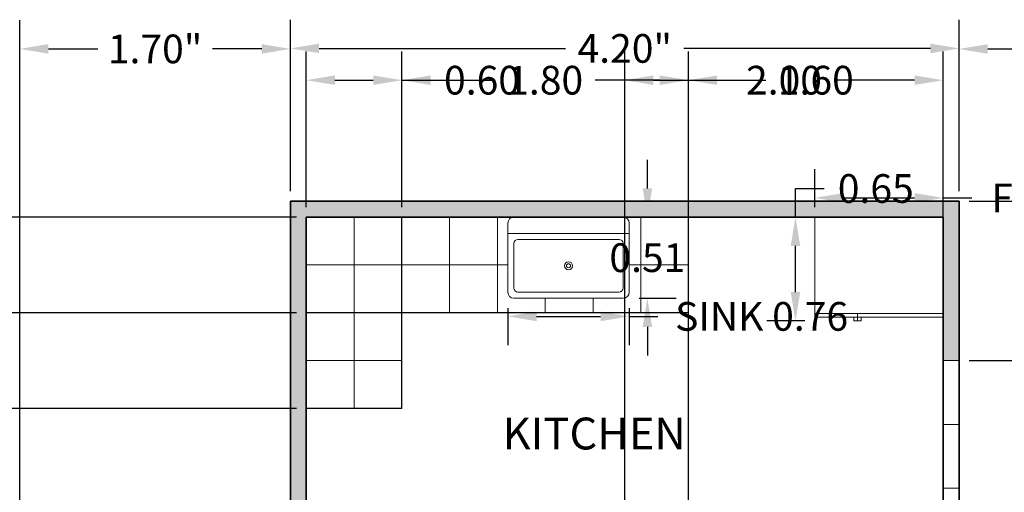
# Model space of a CAD drawing. Units: metres. Extents: x -1.9 to 13.1, y 0.9 to 14.8.
# Tile 6 of 7: x 1.2 to 7.4, y 11.9 to 14.8. Entities that reach past the tile are written whole.
import ezdxf

# ---------------------------------------------------------------- set-up
doc = ezdxf.new("R2010")
doc.units = ezdxf.units.M
doc.header["$MEASUREMENT"] = 0
for name, color, linetype, lineweight in [('A-ANNO-DIMS', 2, 'Continuous', 13), ('A-AREA-IDEN', 7, 'Continuous', 25), ('A-EQPM', 8, 'Continuous', 18), ('A-FLOR-CASE', 8, 'Continuous', 25), ('A-FLOR-FIXT', 8, 'Continuous', 18), ('A-FLOR-PATT', 9, 'Continuous', 13), ('A-GLAZ', 4, 'Continuous', 18), ('A-WALL', 7, 'Continuous', 35), ('A-WALL-PATT', 252, 'Continuous', 13)]:
    doc.layers.add(name, color=color, linetype=linetype, lineweight=lineweight)
doc.styles.get("Standard").update_dxf_attribs({"font": 'arial.ttf'})
doc.dimstyles.get("Standard").update_dxf_attribs({"dimtxt": 0.18, "dimasz": 0.18, "dimexe": 0.18, "dimexo": 0.0625, "dimgap": 0.09, "dimtad": 0, "dimtih": 1, "dimtoh": 1, "dimzin": 0, "dimdsep": 46, "dimlunit": 3, "dimtxsty": 'Standard', "dimcen": 0.09, "dimadec": 0, "dimazin": 0, "dimtfac": 1, "dimtofl": 0, "dimtmove": 0, "dimatfit": 3, "dimfxl": 1, "dimtolj": 1, "dimtzin": 0, "dimarcsym": 0})

# ---------------------------------------------------------------- blocks, each defined once
blk = doc.blocks.new('Refrigerator-2 door - 36 in top')
for p, q in [((0, -26.999999), (36, -26.999999)), ((12, -26.999999), (12, -28.999999)), ((11, -27.999999), (11, -28.999999)), ((11, -28.999999), (13, -28.999999)), ((13, -28.999999), (13, -27.999999))]:
    blk.add_line(p, q)
blk.add_lwpolyline([(0, -27.999999), (0, 0), (36, 0), (36, -27.999999)], close=True)
blk = doc.blocks.new('Sink-single - 30 in top')
blk.add_line((-15, -3.999996), (15, -3.999996))
for points in [[(-13.5, 0), (13.5, 0)], [(-15, -18.499996), (-15, -1.5)], [(15, -1.5), (15, -18.499996)], [(-13.5, -17.499996), (-13.5, -6.499996)], [(-12.5, -5.499996), (12.5, -5.499996)], [(13.5, -6.499996), (13.5, -17.499996)], [(12.5, -18.499996), (-12.5, -18.499996)], [(13.5, -19.999996), (-13.5, -19.999996)]]:
    blk.add_lwpolyline(points)
for radius in [1, 0.5]:
    blk.add_circle((0, -11.999996), radius)
for centre, radius, start, end in [((-13.5, -1.5), 1.5, 90, 180), ((13.5, -1.5), 1.5, 0, 90), ((-12.5, -6.499996), 1, 90, 180), ((12.5, -6.499996), 1, 0, 90), ((-13.5, -18.499996), 1.5, 180, 270), ((-12.5, -17.499996), 1, 180, 270), ((12.5, -17.499996), 1, 270, 0), ((13.5, -18.499996), 1.5, 270, 0)]:
    blk.add_arc(centre, radius, start, end)
blk = doc.blocks.new('*D13')
at = {"layer": 'A-ANNO-DIMS', "color": 0, "lineweight": -2, "transparency": 16777216}
for p, q in [((7.1663, 13.6964), (12.9272, 13.6964)), ((12.7472, 13.5164), (12.7472, 8.3783)), ((12.7472, 2.8764), (12.7472, 8.0145)), ((10.2663, 2.6964), (12.9272, 2.6964))]:
    blk.add_line(p, q, dxfattribs=at)
at = {"layer": 'A-ANNO-DIMS', "color": 0, "transparency": 16777216}
for points in [[(12.7172, 13.5164), (12.7772, 13.5164), (12.7472, 13.6964)], [(12.7172, 2.8764), (12.7772, 2.8764), (12.7472, 2.6964)]]:
    blk.add_solid(points, dxfattribs=at)
at = {"layer": 'Defpoints', "color": 0, "transparency": 16777216}
for p in [(7.1038, 13.6964), (12.7472, 13.6964), (10.2038, 2.6964)]:
    blk.add_point(p, dxfattribs=at)
at = {"layer": 'A-ANNO-DIMS', "color": 0, "transparency": 16777216, "insert": (12.7472, 8.1964), "char_height": 0.18, "attachment_point": 5}
blk.add_mtext('\\A1;11.00"', dxfattribs=at)
blk = doc.blocks.new('*D16')
at = {"layer": 'A-ANNO-DIMS', "color": 0, "lineweight": -2, "transparency": 16777216}
for p, q in [((7.1663, 13.6964), (11.6482, 13.6964)), ((11.4682, 13.5164), (11.4682, 12.3283)), ((11.4682, 10.7764), (11.4682, 11.9644)), ((7.1663, 10.5964), (11.6482, 10.5964))]:
    blk.add_line(p, q, dxfattribs=at)
at = {"layer": 'A-ANNO-DIMS', "color": 0, "transparency": 16777216}
for points in [[(11.4382, 13.5164), (11.4982, 13.5164), (11.4682, 13.6964)], [(11.4382, 10.7764), (11.4982, 10.7764), (11.4682, 10.5964)]]:
    blk.add_solid(points, dxfattribs=at)
at = {"layer": 'Defpoints', "color": 0, "transparency": 16777216}
for p in [(7.1038, 13.6964), (11.4682, 13.6964), (7.1038, 10.5964)]:
    blk.add_point(p, dxfattribs=at)
at = {"layer": 'A-ANNO-DIMS', "color": 0, "transparency": 16777216, "insert": (11.4682, 12.1464), "char_height": 0.18, "attachment_point": 5}
blk.add_mtext('\\A1;3.10"', dxfattribs=at)
blk = doc.blocks.new('*D17')
at = {"layer": 'A-ANNO-DIMS', "color": 0, "lineweight": -2, "transparency": 16777216}
for p, q in [((7.1038, 13.7589), (7.1038, 14.8315)), ((10.2038, 10.6589), (10.2038, 14.8315)), ((7.2838, 14.6515), (8.2857, 14.6515)), ((10.0238, 14.6515), (9.022, 14.6515))]:
    blk.add_line(p, q, dxfattribs=at)
at = {"layer": 'A-ANNO-DIMS', "color": 0, "transparency": 16777216}
for points in [[(7.2838, 14.6815), (7.2838, 14.6215), (7.1038, 14.6515)], [(10.0238, 14.6815), (10.0238, 14.6215), (10.2038, 14.6515)]]:
    blk.add_solid(points, dxfattribs=at)
at = {"layer": 'Defpoints', "color": 0, "transparency": 16777216}
for p in [(7.1038, 14.6515), (7.1038, 13.6964), (10.2038, 10.5964)]:
    blk.add_point(p, dxfattribs=at)
at = {"layer": 'A-ANNO-DIMS', "color": 0, "transparency": 16777216, "insert": (8.6538, 14.6515), "char_height": 0.18, "attachment_point": 5}
blk.add_mtext('\\A1;3.10"', dxfattribs=at)
blk = doc.blocks.new('*D18')
at = {"layer": 'A-ANNO-DIMS', "color": 0, "lineweight": -2, "transparency": 16777216}
for p, q in [((2.9038, 13.7589), (2.9038, 14.8352)), ((7.1038, 13.7589), (7.1038, 14.8352)), ((3.0838, 14.6552), (4.632, 14.6552)), ((6.9238, 14.6552), (5.3757, 14.6552))]:
    blk.add_line(p, q, dxfattribs=at)
at = {"layer": 'A-ANNO-DIMS', "color": 0, "transparency": 16777216}
for points in [[(3.0838, 14.6852), (3.0838, 14.6252), (2.9038, 14.6552)], [(6.9238, 14.6852), (6.9238, 14.6252), (7.1038, 14.6552)]]:
    blk.add_solid(points, dxfattribs=at)
at = {"layer": 'Defpoints', "color": 0, "transparency": 16777216}
for p in [(2.9038, 14.6552), (2.9038, 13.6964), (7.1038, 13.6964)]:
    blk.add_point(p, dxfattribs=at)
at = {"layer": 'A-ANNO-DIMS', "color": 0, "transparency": 16777216, "insert": (5.0038, 14.6552), "char_height": 0.18, "attachment_point": 5}
blk.add_mtext('\\A1;4.20"', dxfattribs=at)
blk = doc.blocks.new('*D19')
at = {"layer": 'A-ANNO-DIMS', "color": 0, "lineweight": -2, "transparency": 16777216}
for p, q in [((1.2038, 10.6589), (1.2038, 14.8321)), ((2.9038, 13.7589), (2.9038, 14.8321)), ((1.3838, 14.6521), (1.6941, 14.6521)), ((2.7238, 14.6521), (2.4136, 14.6521))]:
    blk.add_line(p, q, dxfattribs=at)
at = {"layer": 'A-ANNO-DIMS', "color": 0, "transparency": 16777216}
for points in [[(1.3838, 14.6821), (1.3838, 14.6221), (1.2038, 14.6521)], [(2.7238, 14.6821), (2.7238, 14.6221), (2.9038, 14.6521)]]:
    blk.add_solid(points, dxfattribs=at)
at = {"layer": 'Defpoints', "color": 0, "transparency": 16777216}
for p in [(1.2038, 14.6521), (2.9038, 13.6964), (1.2038, 10.5964)]:
    blk.add_point(p, dxfattribs=at)
at = {"layer": 'A-ANNO-DIMS', "color": 0, "transparency": 16777216, "insert": (2.0538, 14.6521), "char_height": 0.18, "attachment_point": 5}
blk.add_mtext('\\A1;1.70"', dxfattribs=at)
blk = doc.blocks.new('*D46')
at = {"layer": 'A-ANNO-DIMS', "color": 0, "lineweight": -2, "transparency": 16777216}
for p, q in [((6.197, 13.6589), (6.197, 13.8974)), ((7.0038, 13.6589), (7.0038, 13.8974)), ((6.377, 13.7174), (6.8238, 13.7174)), ((7.0038, 13.7174), (7.1838, 13.7174))]:
    blk.add_line(p, q, dxfattribs=at)
at = {"layer": 'A-ANNO-DIMS', "color": 0, "transparency": 16777216}
for points in [[(6.377, 13.7474), (6.377, 13.6874), (6.197, 13.7174)], [(6.8238, 13.7474), (6.8238, 13.6874), (7.0038, 13.7174)]]:
    blk.add_solid(points, dxfattribs=at)
at = {"layer": 'Defpoints', "color": 0, "transparency": 16777216}
for p in [(7.0038, 13.7174), (6.197, 13.5964), (7.0038, 13.5964)]:
    blk.add_point(p, dxfattribs=at)
at = {"layer": 'A-ANNO-DIMS', "color": 0, "transparency": 16777216, "insert": (7.9951, 13.7174), "char_height": 0.18, "attachment_point": 5}
blk.add_mtext('\\A1;FRIDGE 0.81', dxfattribs=at)
blk = doc.blocks.new('*D47')
at = {"layer": 'A-ANNO-DIMS', "color": 0, "lineweight": -2, "transparency": 16777216}
for p, q in [((6.0759, 13.5964), (6.0759, 13.7764)), ((6.0759, 13.7764), (6.2559, 13.7764)), ((6.1345, 13.5964), (5.8959, 13.5964)), ((6.0759, 13.1264), (6.0759, 13.4164)), ((6.1345, 12.9464), (5.8959, 12.9464))]:
    blk.add_line(p, q, dxfattribs=at)
at = {"layer": 'A-ANNO-DIMS', "color": 0, "transparency": 16777216}
for points in [[(6.0459, 13.4164), (6.1059, 13.4164), (6.0759, 13.5964)], [(6.0459, 13.1264), (6.1059, 13.1264), (6.0759, 12.9464)]]:
    blk.add_solid(points, dxfattribs=at)
at = {"layer": 'Defpoints', "color": 0, "transparency": 16777216}
for p in [(6.0759, 13.5964), (6.197, 13.5964), (6.197, 12.9464)]:
    blk.add_point(p, dxfattribs=at)
at = {"layer": 'A-ANNO-DIMS', "color": 0, "transparency": 16777216, "insert": (6.5804, 13.7764), "char_height": 0.18, "attachment_point": 5}
blk.add_mtext('\\A1;0.65', dxfattribs=at)
blk = doc.blocks.new('*D48')
at = {"layer": 'A-ANNO-DIMS', "color": 0, "lineweight": -2, "transparency": 16777216}
for p, q in [((4.2696, 13.0259), (4.2696, 12.7941)), ((5.0316, 13.0259), (5.0316, 12.7941)), ((4.4496, 12.9741), (4.8516, 12.9741)), ((5.0316, 12.9741), (5.2116, 12.9741))]:
    blk.add_line(p, q, dxfattribs=at)
at = {"layer": 'A-ANNO-DIMS', "color": 0, "transparency": 16777216}
for points in [[(4.4496, 13.0041), (4.4496, 12.9441), (4.2696, 12.9741)], [(4.8516, 13.0041), (4.8516, 12.9441), (5.0316, 12.9741)]]:
    blk.add_solid(points, dxfattribs=at)
at = {"layer": 'Defpoints', "color": 0, "transparency": 16777216}
for p in [(4.2696, 13.0884), (5.0316, 13.0884), (5.0316, 12.9741)]:
    blk.add_point(p, dxfattribs=at)
at = {"layer": 'A-ANNO-DIMS', "color": 0, "transparency": 16777216, "insert": (5.8633, 12.9741), "char_height": 0.18, "attachment_point": 5}
blk.add_mtext('\\A1;SINK 0.76', dxfattribs=at)
blk = doc.blocks.new('*D49')
at = {"layer": 'A-ANNO-DIMS', "color": 0, "lineweight": -2, "transparency": 16777216}
for p, q in [((5.1459, 13.7764), (5.1459, 13.9564)), ((5.0941, 13.5964), (5.3259, 13.5964)), ((5.0941, 13.0884), (5.3259, 13.0884)), ((5.1459, 12.9084), (5.1459, 12.7284))]:
    blk.add_line(p, q, dxfattribs=at)
at = {"layer": 'A-ANNO-DIMS', "color": 0, "transparency": 16777216}
for points in [[(5.1159, 13.7764), (5.1759, 13.7764), (5.1459, 13.5964)], [(5.1159, 12.9084), (5.1759, 12.9084), (5.1459, 13.0884)]]:
    blk.add_solid(points, dxfattribs=at)
at = {"layer": 'Defpoints', "color": 0, "transparency": 16777216}
for p in [(5.0316, 13.5964), (5.1459, 13.5964), (5.0316, 13.0884)]:
    blk.add_point(p, dxfattribs=at)
at = {"layer": 'A-ANNO-DIMS', "color": 0, "transparency": 16777216, "insert": (5.1459, 13.3424), "char_height": 0.18, "attachment_point": 5}
blk.add_mtext('\\A1;0.51', dxfattribs=at)
blk = doc.blocks.new('*D60')
at = {"layer": 'A-ANNO-DIMS', "color": 0, "lineweight": -2, "transparency": 16777216}
for p, q in [((7.1663, 13.6964), (11.1433, 13.6964)), ((10.9633, 13.5164), (10.9633, 13.3783)), ((10.9633, 12.8764), (10.9633, 13.0145)), ((7.1663, 12.6964), (11.1433, 12.6964))]:
    blk.add_line(p, q, dxfattribs=at)
at = {"layer": 'A-ANNO-DIMS', "color": 0, "transparency": 16777216}
for points in [[(10.9333, 13.5164), (10.9933, 13.5164), (10.9633, 13.6964)], [(10.9333, 12.8764), (10.9933, 12.8764), (10.9633, 12.6964)]]:
    blk.add_solid(points, dxfattribs=at)
at = {"layer": 'Defpoints', "color": 0, "transparency": 16777216}
for p in [(7.1038, 13.6964), (10.9633, 13.6964), (7.1038, 12.6964)]:
    blk.add_point(p, dxfattribs=at)
at = {"layer": 'A-ANNO-DIMS', "color": 0, "transparency": 16777216, "insert": (10.9633, 13.1964), "char_height": 0.18, "attachment_point": 5}
blk.add_mtext('\\A1;1.00', dxfattribs=at)
blk = doc.blocks.new('*D61')
at = {"layer": 'A-ANNO-DIMS', "color": 0, "lineweight": -2, "transparency": 16777216}
for p, q in [((7.1663, 12.6964), (11.1433, 12.6964)), ((10.9633, 12.5164), (10.9633, 12.2783)), ((10.9633, 11.6764), (10.9633, 11.9145)), ((7.1663, 11.4964), (11.1433, 11.4964))]:
    blk.add_line(p, q, dxfattribs=at)
at = {"layer": 'A-ANNO-DIMS', "color": 0, "transparency": 16777216}
for points in [[(10.9333, 12.5164), (10.9933, 12.5164), (10.9633, 12.6964)], [(10.9333, 11.6764), (10.9933, 11.6764), (10.9633, 11.4964)]]:
    blk.add_solid(points, dxfattribs=at)
at = {"layer": 'Defpoints', "color": 0, "transparency": 16777216}
for p in [(7.1038, 12.6964), (7.1038, 11.4964), (10.9633, 11.4964)]:
    blk.add_point(p, dxfattribs=at)
at = {"layer": 'A-ANNO-DIMS', "color": 0, "transparency": 16777216, "insert": (10.9633, 12.0964), "char_height": 0.18, "attachment_point": 5}
blk.add_mtext('\\A1;1.20', dxfattribs=at)
blk = doc.blocks.new('*D66')
at = {"layer": 'A-ANNO-DIMS', "color": 0, "lineweight": -2, "transparency": 16777216}
for p, q in [((5.403847, 4.558878), (5.403847, 14.635878)), ((7.003847, 4.558878), (7.003847, 14.635878)), ((5.583847, 14.455878), (5.888847, 14.455878)), ((6.823847, 14.455878), (6.518847, 14.455878))]:
    blk.add_line(p, q, dxfattribs=at)
at = {"layer": 'A-ANNO-DIMS', "color": 0, "transparency": 16777216}
for points in [[(5.583847, 14.485878), (5.583847, 14.425878), (5.403847, 14.455878)], [(6.823847, 14.485878), (6.823847, 14.425878), (7.003847, 14.455878)]]:
    blk.add_solid(points, dxfattribs=at)
at = {"layer": 'Defpoints', "color": 0, "transparency": 16777216}
for p in [(7.003847, 14.455878), (5.403847, 4.496378), (7.003847, 4.496378)]:
    blk.add_point(p, dxfattribs=at)
at = {"layer": 'A-ANNO-DIMS', "color": 0, "transparency": 16777216, "insert": (6.203847, 14.455878), "char_height": 0.18, "attachment_point": 5}
blk.add_mtext('\\A1;1.60', dxfattribs=at)
blk = doc.blocks.new('*D69')
at = {"layer": 'A-ANNO-DIMS', "color": 0, "lineweight": -2, "transparency": 16777216}
for p, q in [((3.603847, 13.658878), (3.603847, 14.635878)), ((5.403847, 13.658878), (5.403847, 14.635878)), ((3.783847, 14.455878), (4.188847, 14.455878)), ((5.223847, 14.455878), (4.818847, 14.455878))]:
    blk.add_line(p, q, dxfattribs=at)
at = {"layer": 'A-ANNO-DIMS', "color": 0, "transparency": 16777216}
for points in [[(3.783847, 14.485878), (3.783847, 14.425878), (3.603847, 14.455878)], [(5.223847, 14.485878), (5.223847, 14.425878), (5.403847, 14.455878)]]:
    blk.add_solid(points, dxfattribs=at)
at = {"layer": 'Defpoints', "color": 0, "transparency": 16777216}
for p in [(5.403847, 14.455878), (3.603847, 13.596378), (5.403847, 13.596378)]:
    blk.add_point(p, dxfattribs=at)
at = {"layer": 'A-ANNO-DIMS', "color": 0, "transparency": 16777216, "insert": (4.503847, 14.455878), "char_height": 0.18, "attachment_point": 5}
blk.add_mtext('\\A1;1.80', dxfattribs=at)
blk = doc.blocks.new('*D70')
at = {"layer": 'A-ANNO-DIMS', "color": 0, "lineweight": -2, "transparency": 16777216}
for p, q in [((3.0038, 13.6589), (3.0038, 14.6359)), ((3.6038, 13.6589), (3.6038, 14.6359)), ((3.1838, 14.4559), (3.4238, 14.4559)), ((3.6038, 14.4559), (3.7838, 14.4559))]:
    blk.add_line(p, q, dxfattribs=at)
at = {"layer": 'A-ANNO-DIMS', "color": 0, "transparency": 16777216}
for points in [[(3.1838, 14.4859), (3.1838, 14.4259), (3.0038, 14.4559)], [(3.4238, 14.4859), (3.4238, 14.4259), (3.6038, 14.4559)]]:
    blk.add_solid(points, dxfattribs=at)
at = {"layer": 'Defpoints', "color": 0, "transparency": 16777216}
for p in [(3.6038, 14.4559), (3.0038, 13.5964), (3.6038, 13.5964)]:
    blk.add_point(p, dxfattribs=at)
at = {"layer": 'A-ANNO-DIMS', "color": 0, "transparency": 16777216, "insert": (4.1073, 14.4559), "char_height": 0.18, "attachment_point": 5}
blk.add_mtext('\\A1;0.60', dxfattribs=at)
blk = doc.blocks.new('*D71')
at = {"layer": 'A-ANNO-DIMS', "color": 0, "lineweight": -2, "transparency": 16777216}
for p, q in [((2.9413, 13.5964), (0.2643, 13.5964)), ((0.4443, 13.4164), (0.4443, 13.1764)), ((2.9413, 12.9964), (0.2643, 12.9964)), ((0.4443, 12.9964), (0.4443, 12.8164)), ((0.4443, 12.8164), (0.2643, 12.8164))]:
    blk.add_line(p, q, dxfattribs=at)
at = {"layer": 'A-ANNO-DIMS', "color": 0, "transparency": 16777216}
for points in [[(0.4143, 13.4164), (0.4743, 13.4164), (0.4443, 13.5964)], [(0.4143, 13.1764), (0.4743, 13.1764), (0.4443, 12.9964)]]:
    blk.add_solid(points, dxfattribs=at)
at = {"layer": 'Defpoints', "color": 0, "transparency": 16777216}
for p in [(3.0038, 13.5964), (0.4443, 12.9964), (3.0038, 12.9964)]:
    blk.add_point(p, dxfattribs=at)
at = {"layer": 'A-ANNO-DIMS', "color": 0, "transparency": 16777216, "insert": (-0.0591, 12.8164), "char_height": 0.18, "attachment_point": 5}
blk.add_mtext('\\A1;0.60', dxfattribs=at)
blk = doc.blocks.new('*D72')
at = {"layer": 'A-ANNO-DIMS', "color": 0, "lineweight": -2, "transparency": 16777216}
for p, q in [((2.9413, 12.9964), (0.2643, 12.9964)), ((0.4443, 12.8164), (0.4443, 12.5764)), ((2.9413, 12.3964), (0.2643, 12.3964)), ((0.4443, 12.3964), (0.4443, 12.2164)), ((0.4443, 12.2164), (0.2643, 12.2164))]:
    blk.add_line(p, q, dxfattribs=at)
at = {"layer": 'A-ANNO-DIMS', "color": 0, "transparency": 16777216}
for points in [[(0.4143, 12.8164), (0.4743, 12.8164), (0.4443, 12.9964)], [(0.4143, 12.5764), (0.4743, 12.5764), (0.4443, 12.3964)]]:
    blk.add_solid(points, dxfattribs=at)
at = {"layer": 'Defpoints', "color": 0, "transparency": 16777216}
for p in [(3.0038, 12.9964), (0.4443, 12.3964), (3.0038, 12.3964)]:
    blk.add_point(p, dxfattribs=at)
at = {"layer": 'A-ANNO-DIMS', "color": 0, "transparency": 16777216, "insert": (-0.0591, 12.2164), "char_height": 0.18, "attachment_point": 5}
blk.add_mtext('\\A1;0.60', dxfattribs=at)
blk = doc.blocks.new('*D73')
at = {"layer": 'A-ANNO-DIMS', "color": 0, "lineweight": -2, "transparency": 16777216}
for p, q in [((5.0038, 10.6589), (5.0038, 14.6359)), ((7.0038, 9.2589), (7.0038, 14.6359)), ((5.1838, 14.4559), (5.6788, 14.4559)), ((6.8238, 14.4559), (6.3289, 14.4559))]:
    blk.add_line(p, q, dxfattribs=at)
at = {"layer": 'A-ANNO-DIMS', "color": 0, "transparency": 16777216}
for points in [[(5.1838, 14.4859), (5.1838, 14.4259), (5.0038, 14.4559)], [(6.8238, 14.4859), (6.8238, 14.4259), (7.0038, 14.4559)]]:
    blk.add_solid(points, dxfattribs=at)
at = {"layer": 'Defpoints', "color": 0, "transparency": 16777216}
for p in [(7.0038, 14.4559), (5.0038, 10.5964), (7.0038, 9.1964)]:
    blk.add_point(p, dxfattribs=at)
at = {"layer": 'A-ANNO-DIMS', "color": 0, "transparency": 16777216, "insert": (6.0038, 14.4559), "char_height": 0.18, "attachment_point": 5}
blk.add_mtext('\\A1;2.00', dxfattribs=at)

msp = doc.modelspace()

# ---------------------------------------------------------------- hatches: boundary and pattern name
at = {"layer": 'A-FLOR-PATT'}
h = msp.add_hatch(dxfattribs=at)
h.set_pattern_fill('ANSI31', color=256, scale=2.4028, angle=45, style=0)
h.paths.add_polyline_path([(3.0038, 12.3964), (3.6038, 12.3964), (3.6038, 13.5964), (3.0038, 13.5964)])
h = msp.add_hatch(dxfattribs=at)
h.set_pattern_fill('ANSI31', color=256, scale=2.4175, angle=-45, style=0)
h.paths.add_polyline_path([(3.0038, 12.9964), (5.4038, 12.9964), (5.4038, 13.5964), (5.0316, 13.5964), (5.0316, 13.0884), (4.2696, 13.0884), (4.2696, 13.5964), (3.0038, 13.5964)])
h = msp.add_hatch(dxfattribs=at)
h.set_pattern_fill('ANSI31', color=256, scale=2.4021, angle=45, style=0)
h.paths.add_polyline_path([(3.6038, 12.9964), (5.4038, 12.9964), (5.4038, 13.5964), (5.0316, 13.5964), (5.0316, 13.0884), (4.2696, 13.0884), (4.2696, 13.5964), (3.6038, 13.5964)])
h = msp.add_hatch(dxfattribs=at)
h.set_pattern_fill('ANSI31', color=256, scale=2.4184, angle=-45, style=0)
h.paths.add_polyline_path([(3.0038, 12.3964), (3.6038, 12.3964), (3.6038, 12.9964), (3.0038, 12.9964)])

# ---------------------------------------------------------------- linework, layer by layer
at = {"layer": 'A-FLOR-CASE'}
for p, q in [((3.6038, 12.3964), (3.6038, 13.5964)), ((5.4038, 12.9964), (5.4038, 13.5964)), ((5.4038, 12.9964), (3.0038, 12.9964)), ((3.6038, 12.3964), (3.0038, 12.3964))]:
    msp.add_line(p, q, dxfattribs=at)
at = {"layer": 'A-GLAZ'}
for p, q in [((7.1038, 12.6964), (7.0038, 12.6964)), ((7.1038, 12.2964), (7.0038, 12.2964)), ((7.1038, 11.8964), (7.0038, 11.8964))]:
    msp.add_line(p, q, dxfattribs=at)
at = {"layer": 'A-WALL'}
for p, q in [((2.9038, 11.3964), (2.9038, 13.6964)), ((7.1038, 10.5964), (7.1038, 13.6964)), ((7.0038, 13.5964), (3.0038, 13.5964)), ((3.0038, 11.3964), (3.0038, 13.5964)), ((7.0038, 9.1964), (7.0038, 13.5964))]:
    msp.add_line(p, q, dxfattribs=at)
msp.add_lwpolyline([(7.1038, 13.6964), (2.9038, 13.6964)], dxfattribs=at)
at = {"layer": 'A-WALL-PATT'}
for points in [[(2.9038, 11.3964), (3.0038, 11.3964), (2.9038, 13.6964), (3.0038, 13.5964)], [(2.9038, 13.6964), (3.0038, 13.5964), (7.1038, 13.6964), (7.0038, 13.5964)], [(7.1038, 13.6964), (7.0038, 13.5964), (7.1038, 12.6964), (7.0038, 12.6964)]]:
    msp.add_solid(points, dxfattribs=at)

# ---------------------------------------------------------------- block references
at = {"layer": 'A-EQPM', "xscale": 0.0224134950046578, "yscale": 0.0224134950046578, "zscale": 0.0224134950046578}
msp.add_blockref('Refrigerator-2 door - 36 in top', (6.197, 13.5964), dxfattribs=at)
at = {"layer": 'A-FLOR-FIXT', "xscale": 0.0254, "yscale": 0.0254, "zscale": 0.0254}
msp.add_blockref('Sink-single - 30 in top', (4.6506, 13.5964), dxfattribs=at)

# ---------------------------------------------------------------- texts
at = {"layer": 'A-AREA-IDEN', "insert": (4.1691, 12.3392), "char_height": 0.2, "attachment_point": 1}
msp.add_mtext_dynamic_manual_height_columns('\\pxqc;KITCHEN', width=1.285752, gutter_width=1, heights=[0], dxfattribs=at)

# ---------------------------------------------------------------- dimensions: what is measured, and where the dimension line sits
at = {"layer": 'A-ANNO-DIMS'}
for base, p1, p2, override, picture, middle in [((1.2038, 14.6521), (2.9038, 13.6964), (1.2038, 10.5964), {"dimclrd": 0, "dimclre": 0, "dimclrt": 0}, '*D19', (2.0538, 14.6521)), ((2.9038, 14.6552), (7.1038, 13.6964), (2.9038, 13.6964), {"dimclrd": 0, "dimclre": 0, "dimclrt": 0}, '*D18', (5.0038, 14.6552)), ((7.1038, 14.6515), (10.2038, 10.5964), (7.1038, 13.6964), {"dimclrd": 0, "dimclre": 0, "dimclrt": 0}, '*D17', (8.6538, 14.6515)), ((3.6038, 14.4559), (3.0038, 13.5964), (3.6038, 13.5964), {"dimdec": 2, "dimlfac": 1, "dimrnd": 0, "dimzin": 0, "dimdsep": 46, "dimlunit": 2}, '*D70', (4.1073, 14.4559)), ((5.4038, 14.4559), (3.6038, 13.5964), (5.4038, 13.5964), {"dimdec": 2, "dimlfac": 1, "dimrnd": 0, "dimzin": 0, "dimdsep": 46, "dimlunit": 2}, '*D69', (4.5038, 14.4559)), ((7.0038, 14.4559), (5.0038, 10.5964), (7.0038, 9.1964), {"dimdec": 2, "dimlfac": 1, "dimrnd": 0, "dimzin": 0, "dimdsep": 46, "dimlunit": 2}, '*D73', (6.0038, 14.4559)), ((7.0038, 14.4559), (5.4038, 4.4964), (7.0038, 4.4964), {"dimdec": 2, "dimlfac": 1, "dimrnd": 0, "dimzin": 0, "dimdsep": 46, "dimlunit": 2}, '*D66', (6.2038, 14.4559))]:
    dim = msp.add_linear_dim(base=base, p1=p1, p2=p2, dimstyle='Standard', override=override, dxfattribs=at)
    dim.commit()
    dim.dimension.update_dxf_attribs({"geometry": picture, "text_midpoint": middle})
for base, p1, p2, text, picture, middle in [((7.0038, 13.7174), (6.197, 13.5964), (7.0038, 13.5964), 'FRIDGE <>', '*D46', (7.9951, 13.7174)), ((5.0316, 12.9741), (4.2696, 13.0884), (5.0316, 13.0884), 'SINK <>', '*D48', (5.8633, 12.9741))]:
    dim = msp.add_linear_dim(base=base, p1=p1, p2=p2, text=text, dimstyle='Standard', override={"dimdec": 2, "dimlfac": 1, "dimrnd": 0, "dimzin": 0, "dimdsep": 46, "dimlunit": 2}, dxfattribs=at)
    dim.commit()
    dim.dimension.update_dxf_attribs({"geometry": picture, "text_midpoint": middle})
for base, p1, p2, override, picture, middle in [((5.1459, 13.5964), (5.0316, 13.0884), (5.0316, 13.5964), {"dimdec": 2, "dimlfac": 1, "dimrnd": 0, "dimzin": 0, "dimdsep": 46, "dimlunit": 2}, '*D49', (5.1459, 13.3424)), ((6.0759, 13.5964), (6.197, 12.9464), (6.197, 13.5964), {"dimdec": 2, "dimlfac": 1, "dimrnd": 0, "dimzin": 0, "dimdsep": 46, "dimlunit": 2}, '*D47', (6.5804, 13.7764)), ((12.7472, 13.6964), (10.2038, 2.6964), (7.1038, 13.6964), {"dimclrd": 0, "dimclre": 0, "dimclrt": 0}, '*D13', (12.7472, 8.1964)), ((11.4682, 13.6964), (7.1038, 10.5964), (7.1038, 13.6964), {"dimclrd": 0, "dimclre": 0, "dimclrt": 0}, '*D16', (11.4682, 12.1464)), ((10.9633, 13.6964), (7.1038, 12.6964), (7.1038, 13.6964), {"dimdec": 2, "dimlfac": 1, "dimrnd": 0, "dimzin": 0, "dimdsep": 46, "dimlunit": 2}, '*D60', (10.9633, 13.1964)), ((0.4443, 12.9964), (3.0038, 13.5964), (3.0038, 12.9964), {"dimdec": 2, "dimlfac": 1, "dimrnd": 0, "dimzin": 0, "dimdsep": 46, "dimlunit": 2}, '*D71', (-0.0591, 12.8164)), ((0.4443, 12.3964), (3.0038, 12.9964), (3.0038, 12.3964), {"dimdec": 2, "dimlfac": 1, "dimrnd": 0, "dimzin": 0, "dimdsep": 46, "dimlunit": 2}, '*D72', (-0.0591, 12.2164)), ((10.9633, 11.4964), (7.1038, 12.6964), (7.1038, 11.4964), {"dimdec": 2, "dimlfac": 1, "dimrnd": 0, "dimzin": 0, "dimdsep": 46, "dimlunit": 2}, '*D61', (10.9633, 12.0964))]:
    dim = msp.add_linear_dim(base=base, p1=p1, p2=p2, angle=90, dimstyle='Standard', override=override, dxfattribs=at)
    dim.commit()
    dim.dimension.update_dxf_attribs({"geometry": picture, "text_midpoint": middle})

doc.saveas('drawing.dxf')
